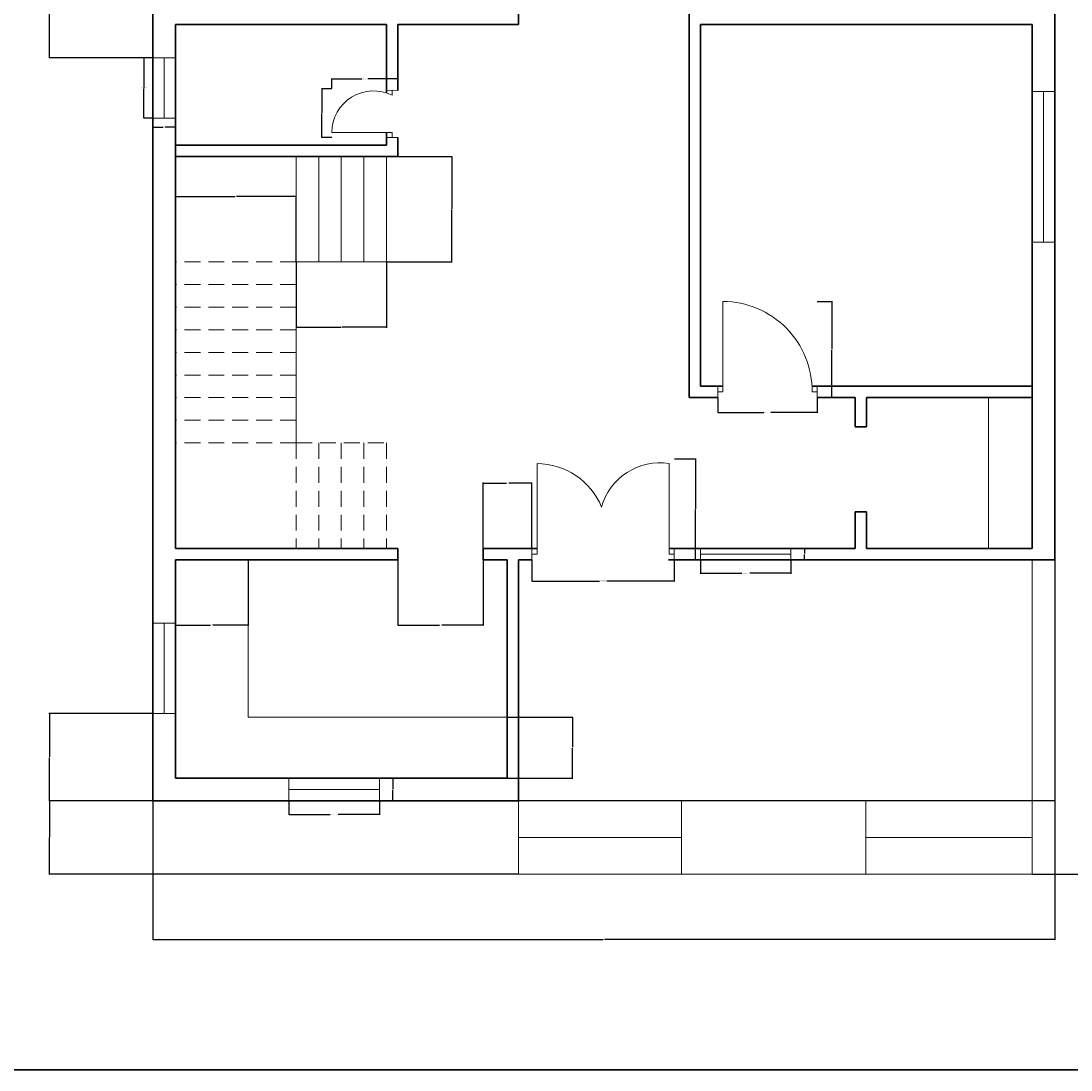
# Model space of a CAD drawing. Units: inches. Extents: x 1832 to 2989, y 1644 to 2902.
# Tile 4 of 8: x 2343 to 2760, y 1644 to 2061. Entities that reach past the tile are written whole.
import ezdxf

# ---------------------------------------------------------------- set-up
doc = ezdxf.new("R2010")
doc.units = ezdxf.units.IN
doc.linetypes.add('DASHED2', pattern=[9.525, 6.35, -3.175])
for name, color, linetype, lineweight in [('A-ANNO-DIMS', 2, 'Continuous', 18), ('A-ANNO-TTLB', 7, 'Continuous', 35), ('A-DOOR', 3, 'Continuous', 18), ('A-FLOR', 7, 'Continuous', 25), ('A-FLOR-CASE', 8, 'Continuous', 18), ('A-FLOR-STRS', 7, 'Continuous', 18), ('A-FLOR-STRS-OVHD', 254, 'DASHED2', 13), ('A-GLAZ', 4, 'Continuous', 18), ('A-WALL', 7, 'Continuous', 35)]:
    doc.layers.add(name, color=color, linetype=linetype, lineweight=lineweight)
doc.styles.get("Standard").update_dxf_attribs({"font": 'arial.ttf'})
doc.dimstyles.get("Standard").update_dxf_attribs({"dimtxt": 0.18, "dimasz": 0.18, "dimexe": 0.18, "dimexo": 0.0625, "dimgap": 0.09, "dimtad": 0, "dimtih": 1, "dimtoh": 1, "dimdec": 4, "dimzin": 0, "dimdsep": 46, "dimtxsty": 'Standard', "dimcen": 0.09, "dimadec": 0, "dimazin": 0, "dimtfac": 1, "dimtdec": 4, "dimtofl": 0, "dimtmove": 0, "dimatfit": 3, "dimfxl": 1, "dimtolj": 1, "dimtzin": 0, "dimarcsym": 0})

# ---------------------------------------------------------------- blocks, each defined once
blk = doc.blocks.new('WIN-PLAN-60IN')
for p, q in [((0, 9), (0, 0)), ((60, 4.5), (60, 9)), ((60, 9), (60, 0)), ((0, 0), (0, 4.5)), ((0, 4.5), (60, 4.5))]:
    blk.add_line(p, q)
blk = doc.blocks.new('WIN-PLAN-24IN')
for p, q in [((0, 9), (0, 0)), ((24, 4.5), (24, 9)), ((24, 9), (24, 0)), ((0, 0), (0, 4.5)), ((0, 4.5), (24, 4.5))]:
    blk.add_line(p, q)
blk = doc.blocks.new('WIN-PLAN-36IN')
for p, q in [((0, 9), (0, 0)), ((36, 4.5), (36, 9)), ((36, 9), (36, 0)), ((0, 0), (0, 4.5)), ((0, 4.5), (36, 4.5))]:
    blk.add_line(p, q)
blk = doc.blocks.new('WIN-PLAN-36IN-2')
for p, q in [((0, 36), (9, 36)), ((9, 36), (4.5, 36)), ((4.5, 36), (4.5, 0)), ((9, 0), (0, 0)), ((4.5, 0), (9, 0))]:
    blk.add_line(p, q)
blk = doc.blocks.new('DOOR-PLAN-WC')
for p, q in [((21.75, 18.87), (26.25, 18.72)), ((26.25, 18.72), (24, 18.8)), ((24, 18.8), (24, 16.8)), ((24, 2), (0, 2)), ((21.75, 0), (26.25, 0)), ((24, 0), (24, 2)), ((26.25, 0), (24, 0))]:
    blk.add_line(p, q)
blk.add_arc((16.56, 2), 16.56, 63.308, 180)
blk = doc.blocks.new('DOOR-PLAN-ENTRY-PAIR')
for p, q in [((2, 2.25), (2, 38.25)), ((54.64, 2.25), (54.64, 38.25)), ((0, 4.5), (0, 0)), ((56.64, 4.5), (56.64, 0)), ((56.64, 4.5), (56.64, 2.25)), ((0, 2.25), (2, 2.25)), ((56.64, 2.25), (54.64, 2.25)), ((56.64, 0), (56.64, 2.25))]:
    blk.add_line(p, q)
for centre, radius, start, end in [((2, 10.56), 27.69, 21.9895, 90), ((50.82, 14.55), 24, 80.8436, 164.5954)]:
    blk.add_arc(centre, radius, start, end)
blk = doc.blocks.new('DOOR-PLAN-LIVING')
for p, q in [((2, 26.25), (2, 38.25)), ((2, 2.25), (2, 26.25)), ((0, 4.5), (0, 0)), ((39.53, 4.5), (39.53, 0)), ((0, 0), (0, 2.25)), ((0, 2.25), (2, 2.25)), ((39.53, 2.25), (37.53, 2.25)), ((39.53, 0), (39.53, 2.25))]:
    blk.add_line(p, q)
blk.add_arc((2, 2.72), 35.53, 359.2416, 90)
blk = doc.blocks.new('WIN-PLAN-PARTITION-36IN')
for p, q in [((0, 4.5), (0, 0)), ((36, 2.25), (36, 4.5)), ((36, 4.5), (36, 0)), ((0, 2.25), (36, 2.25))]:
    blk.add_line(p, q)
blk = doc.blocks.new('*D43')
at = {"layer": 'A-ANNO-DIMS', "color": 0, "lineweight": -2, "transparency": 16777216}
for p, q in [((2466.29, 2034.14), (2466.29, 2038.19)), ((2466.47, 2038.01), (2478.22, 2038.01)), ((2492.36, 2038.01), (2480.6, 2038.01)), ((2492.54, 2034.14), (2492.54, 2038.19))]:
    blk.add_line(p, q, dxfattribs=at)
at = {"layer": 'A-ANNO-DIMS', "color": 0, "transparency": 16777216}
for points in [[(2466.47, 2038.04), (2466.47, 2037.98), (2466.29, 2038.01)], [(2492.36, 2038.04), (2492.36, 2037.98), (2492.54, 2038.01)]]:
    blk.add_solid(points, dxfattribs=at)
at = {"layer": 'Defpoints', "color": 0, "transparency": 16777216}
for p in [(2492.54, 2038.01), (2466.29, 2034.08), (2492.54, 2034.08)]:
    blk.add_point(p, dxfattribs=at)
at = {"layer": 'A-ANNO-DIMS', "color": 0, "transparency": 16777216, "insert": (2479.41, 2038.01), "char_height": 0.18, "attachment_point": 5}
blk.add_mtext('\\A1;WC DOOR 26 TYP.', dxfattribs=at)
blk = doc.blocks.new('*D44')
at = {"layer": 'A-ANNO-DIMS', "color": 0, "lineweight": -2, "transparency": 16777216}
for p, q in [((2466.22, 2034.08), (2462.17, 2034.08)), ((2462.35, 2033.9), (2462.35, 2024.57)), ((2462.35, 2014.88), (2462.35, 2024.21)), ((2466.22, 2014.7), (2462.17, 2014.7))]:
    blk.add_line(p, q, dxfattribs=at)
at = {"layer": 'A-ANNO-DIMS', "color": 0, "transparency": 16777216}
for points in [[(2462.32, 2033.9), (2462.38, 2033.9), (2462.35, 2034.08)], [(2462.32, 2014.88), (2462.38, 2014.88), (2462.35, 2014.7)]]:
    blk.add_solid(points, dxfattribs=at)
at = {"layer": 'Defpoints', "color": 0, "transparency": 16777216}
for p in [(2462.35, 2034.08), (2466.29, 2034.08), (2466.29, 2014.7)]:
    blk.add_point(p, dxfattribs=at)
at = {"layer": 'A-ANNO-DIMS', "color": 0, "transparency": 16777216, "insert": (2462.35, 2024.39), "char_height": 0.18, "attachment_point": 5}
blk.add_mtext('\\A1;19 TYP.', dxfattribs=at)
blk = doc.blocks.new('*D45')
at = {"layer": 'A-ANNO-DIMS', "color": 0, "lineweight": -2, "transparency": 16777216}
for p, q in [((2619.9, 1911.11), (2619.9, 1905.06)), ((2659.42, 1911.11), (2659.42, 1905.06)), ((2620.08, 1905.24), (2638.28, 1905.24)), ((2659.24, 1905.24), (2641.04, 1905.24))]:
    blk.add_line(p, q, dxfattribs=at)
at = {"layer": 'A-ANNO-DIMS', "color": 0, "transparency": 16777216}
for points in [[(2620.08, 1905.27), (2620.08, 1905.21), (2619.9, 1905.24)], [(2659.24, 1905.27), (2659.24, 1905.21), (2659.42, 1905.24)]]:
    blk.add_solid(points, dxfattribs=at)
at = {"layer": 'Defpoints', "color": 0, "transparency": 16777216}
for p in [(2619.9, 1911.17), (2659.42, 1911.17), (2659.42, 1905.24)]:
    blk.add_point(p, dxfattribs=at)
at = {"layer": 'A-ANNO-DIMS', "color": 0, "transparency": 16777216, "insert": (2639.66, 1905.24), "char_height": 0.18, "attachment_point": 5}
blk.add_mtext('\\A1;LIVING DOOR 40 TYP.', dxfattribs=at)
blk = doc.blocks.new('*D46')
at = {"layer": 'A-ANNO-DIMS', "color": 0, "lineweight": -2, "transparency": 16777216}
for p, q in [((2659.49, 1949.42), (2665.53, 1949.42)), ((2665.35, 1949.24), (2665.35, 1930.48)), ((2665.35, 1911.35), (2665.35, 1930.12)), ((2659.49, 1911.17), (2665.53, 1911.17))]:
    blk.add_line(p, q, dxfattribs=at)
at = {"layer": 'A-ANNO-DIMS', "color": 0, "transparency": 16777216}
for points in [[(2665.32, 1949.24), (2665.38, 1949.24), (2665.35, 1949.42)], [(2665.32, 1911.35), (2665.38, 1911.35), (2665.35, 1911.17)]]:
    blk.add_solid(points, dxfattribs=at)
at = {"layer": 'Defpoints', "color": 0, "transparency": 16777216}
for p in [(2659.42, 1949.42), (2665.35, 1949.42), (2659.42, 1911.17)]:
    blk.add_point(p, dxfattribs=at)
at = {"layer": 'A-ANNO-DIMS', "color": 0, "transparency": 16777216, "insert": (2665.35, 1930.3), "char_height": 0.18, "attachment_point": 5}
blk.add_mtext('\\A1;38 TYP.', dxfattribs=at)
blk = doc.blocks.new('*D47')
at = {"layer": 'A-ANNO-DIMS', "color": 0, "lineweight": -2, "transparency": 16777216}
for p, q in [((2545.94, 1846.61), (2545.94, 1838)), ((2602.58, 1846.61), (2602.58, 1838)), ((2546.12, 1838.18), (2572.77, 1838.18)), ((2602.4, 1838.18), (2575.75, 1838.18))]:
    blk.add_line(p, q, dxfattribs=at)
at = {"layer": 'A-ANNO-DIMS', "color": 0, "transparency": 16777216}
for points in [[(2546.12, 1838.21), (2546.12, 1838.15), (2545.94, 1838.18)], [(2602.4, 1838.21), (2602.4, 1838.15), (2602.58, 1838.18)]]:
    blk.add_solid(points, dxfattribs=at)
at = {"layer": 'Defpoints', "color": 0, "transparency": 16777216}
for p in [(2545.94, 1846.67), (2602.58, 1846.67), (2602.58, 1838.18)]:
    blk.add_point(p, dxfattribs=at)
at = {"layer": 'A-ANNO-DIMS', "color": 0, "transparency": 16777216, "insert": (2574.26, 1838.18), "char_height": 0.18, "attachment_point": 5}
blk.add_mtext('\\A1;PAIRED ENTRY 57 TYP.', dxfattribs=at)
blk = doc.blocks.new('*D48')
at = {"layer": 'A-ANNO-DIMS', "color": 0, "lineweight": -2, "transparency": 16777216}
for p, q in [((2602.64, 1886.87), (2611.26, 1886.87)), ((2611.08, 1886.69), (2611.08, 1866.95)), ((2611.08, 1846.85), (2611.08, 1866.59)), ((2602.64, 1846.67), (2611.26, 1846.67))]:
    blk.add_line(p, q, dxfattribs=at)
at = {"layer": 'A-ANNO-DIMS', "color": 0, "transparency": 16777216}
for points in [[(2611.05, 1886.69), (2611.11, 1886.69), (2611.08, 1886.87)], [(2611.05, 1846.85), (2611.11, 1846.85), (2611.08, 1846.67)]]:
    blk.add_solid(points, dxfattribs=at)
at = {"layer": 'Defpoints', "color": 0, "transparency": 16777216}
for p in [(2602.58, 1886.87), (2611.08, 1886.87), (2602.58, 1846.67)]:
    blk.add_point(p, dxfattribs=at)
at = {"layer": 'A-ANNO-DIMS', "color": 0, "transparency": 16777216, "insert": (2611.08, 1866.77), "char_height": 0.18, "attachment_point": 5}
blk.add_mtext('\\A1;40 TYP.', dxfattribs=at)
blk = doc.blocks.new('*D53')
at = {"layer": 'A-ANNO-DIMS', "color": 0, "lineweight": -2, "transparency": 16777216}
for p, q in [((2394.97, 2046.39), (2391.26, 2046.39)), ((2391.44, 2046.21), (2391.44, 2034.57)), ((2391.44, 2022.57), (2391.44, 2034.2)), ((2394.97, 2022.39), (2391.26, 2022.39))]:
    blk.add_line(p, q, dxfattribs=at)
at = {"layer": 'A-ANNO-DIMS', "color": 0, "transparency": 16777216}
for points in [[(2391.41, 2046.21), (2391.47, 2046.21), (2391.44, 2046.39)], [(2391.41, 2022.57), (2391.47, 2022.57), (2391.44, 2022.39)]]:
    blk.add_solid(points, dxfattribs=at)
at = {"layer": 'Defpoints', "color": 0, "transparency": 16777216}
for p in [(2395.04, 2046.39), (2391.44, 2022.39), (2395.04, 2022.39)]:
    blk.add_point(p, dxfattribs=at)
at = {"layer": 'A-ANNO-DIMS', "color": 0, "transparency": 16777216, "insert": (2391.44, 2034.39), "char_height": 0.18, "attachment_point": 5}
blk.add_mtext('\\A1;WC WINDOW 24 TYP.', dxfattribs=at)
blk = doc.blocks.new('*D54')
at = {"layer": 'A-ANNO-DIMS', "color": 0, "lineweight": -2, "transparency": 16777216}
for p, q in [((2395.04, 2022.32), (2395.04, 2018.61)), ((2395.22, 2018.79), (2399.08, 2018.79)), ((2403.86, 2018.79), (2399.99, 2018.79)), ((2404.04, 2022.32), (2404.04, 2018.61))]:
    blk.add_line(p, q, dxfattribs=at)
at = {"layer": 'A-ANNO-DIMS', "color": 0, "transparency": 16777216}
for points in [[(2395.22, 2018.82), (2395.22, 2018.76), (2395.04, 2018.79)], [(2403.86, 2018.82), (2403.86, 2018.76), (2404.04, 2018.79)]]:
    blk.add_solid(points, dxfattribs=at)
at = {"layer": 'Defpoints', "color": 0, "transparency": 16777216}
for p in [(2395.04, 2022.39), (2404.04, 2022.39), (2404.04, 2018.79)]:
    blk.add_point(p, dxfattribs=at)
at = {"layer": 'A-ANNO-DIMS', "color": 0, "transparency": 16777216, "insert": (2399.54, 2018.79), "char_height": 0.18, "attachment_point": 5}
blk.add_mtext('\\A1;9 TYP.', dxfattribs=at)
blk = doc.blocks.new('*D55')
at = {"layer": 'A-ANNO-DIMS', "color": 0, "lineweight": -2, "transparency": 16777216}
for p, q in [((2449.19, 1750.61), (2449.19, 1745.09)), ((2485.19, 1750.61), (2485.19, 1745.09)), ((2449.37, 1745.27), (2465.61, 1745.27)), ((2485.01, 1745.27), (2468.76, 1745.27))]:
    blk.add_line(p, q, dxfattribs=at)
at = {"layer": 'A-ANNO-DIMS', "color": 0, "transparency": 16777216}
for points in [[(2449.37, 1745.3), (2449.37, 1745.24), (2449.19, 1745.27)], [(2485.01, 1745.3), (2485.01, 1745.24), (2485.19, 1745.27)]]:
    blk.add_solid(points, dxfattribs=at)
at = {"layer": 'Defpoints', "color": 0, "transparency": 16777216}
for p in [(2449.19, 1750.67), (2485.19, 1750.67), (2449.19, 1745.27)]:
    blk.add_point(p, dxfattribs=at)
at = {"layer": 'A-ANNO-DIMS', "color": 0, "transparency": 16777216, "insert": (2467.19, 1745.27), "char_height": 0.18, "attachment_point": 5}
blk.add_mtext('\\A1;FRONT WINDOW 36 TYP.', dxfattribs=at)
blk = doc.blocks.new('*D56')
at = {"layer": 'A-ANNO-DIMS', "color": 0, "lineweight": -2, "transparency": 16777216}
for p, q in [((2485.25, 1759.67), (2490.77, 1759.67)), ((2490.59, 1759.49), (2490.59, 1755.35)), ((2490.59, 1750.85), (2490.59, 1754.99)), ((2485.25, 1750.67), (2490.77, 1750.67))]:
    blk.add_line(p, q, dxfattribs=at)
at = {"layer": 'A-ANNO-DIMS', "color": 0, "transparency": 16777216}
for points in [[(2490.56, 1759.49), (2490.62, 1759.49), (2490.59, 1759.67)], [(2490.56, 1750.85), (2490.62, 1750.85), (2490.59, 1750.67)]]:
    blk.add_solid(points, dxfattribs=at)
at = {"layer": 'Defpoints', "color": 0, "transparency": 16777216}
for p in [(2485.19, 1759.67), (2485.19, 1750.67), (2490.59, 1750.67)]:
    blk.add_point(p, dxfattribs=at)
at = {"layer": 'A-ANNO-DIMS', "color": 0, "transparency": 16777216, "insert": (2490.59, 1755.17), "char_height": 0.18, "attachment_point": 5}
blk.add_mtext('\\A1;9 TYP.', dxfattribs=at)
blk = doc.blocks.new('*D59')
at = {"layer": 'A-ANNO-DIMS', "color": 0, "lineweight": -2, "transparency": 16777216}
for p, q in [((2613.04, 1846.61), (2613.04, 1841.09)), ((2649.04, 1846.61), (2649.04, 1841.09)), ((2613.22, 1841.27), (2629.43, 1841.27)), ((2648.86, 1841.27), (2632.65, 1841.27))]:
    blk.add_line(p, q, dxfattribs=at)
at = {"layer": 'A-ANNO-DIMS', "color": 0, "transparency": 16777216}
for points in [[(2613.22, 1841.3), (2613.22, 1841.24), (2613.04, 1841.27)], [(2648.86, 1841.3), (2648.86, 1841.24), (2649.04, 1841.27)]]:
    blk.add_solid(points, dxfattribs=at)
at = {"layer": 'Defpoints', "color": 0, "transparency": 16777216}
for p in [(2613.04, 1846.67), (2649.04, 1846.67), (2649.04, 1841.27)]:
    blk.add_point(p, dxfattribs=at)
at = {"layer": 'A-ANNO-DIMS', "color": 0, "transparency": 16777216, "insert": (2631.04, 1841.27), "char_height": 0.18, "attachment_point": 5}
blk.add_mtext('\\A1;SITOUT WINDOW 36 TYP.', dxfattribs=at)
blk = doc.blocks.new('*D60')
at = {"layer": 'A-ANNO-DIMS', "color": 0, "lineweight": -2, "transparency": 16777216}
for p, q in [((2649.1, 1851.17), (2654.62, 1851.17)), ((2654.44, 1850.99), (2654.44, 1849.1)), ((2654.44, 1846.85), (2654.44, 1848.74)), ((2649.1, 1846.67), (2654.62, 1846.67))]:
    blk.add_line(p, q, dxfattribs=at)
at = {"layer": 'A-ANNO-DIMS', "color": 0, "transparency": 16777216}
for points in [[(2654.41, 1850.99), (2654.47, 1850.99), (2654.44, 1851.17)], [(2654.41, 1846.85), (2654.47, 1846.85), (2654.44, 1846.67)]]:
    blk.add_solid(points, dxfattribs=at)
at = {"layer": 'Defpoints', "color": 0, "transparency": 16777216}
for p in [(2649.04, 1851.17), (2654.44, 1851.17), (2649.04, 1846.67)]:
    blk.add_point(p, dxfattribs=at)
at = {"layer": 'A-ANNO-DIMS', "color": 0, "transparency": 16777216, "insert": (2654.44, 1848.92), "char_height": 0.18, "attachment_point": 5}
blk.add_mtext('\\A1;5 TYP.', dxfattribs=at)
blk = doc.blocks.new('*D81')
at = {"layer": 'A-ANNO-DIMS', "color": 0, "lineweight": -2, "transparency": 16777216}
for p, q in [((2395.04, 1750.61), (2395.04, 1695.34)), ((2754.04, 1750.61), (2754.04, 1695.34)), ((2395.22, 1695.52), (2574.25, 1695.52)), ((2753.86, 1695.52), (2574.82, 1695.52))]:
    blk.add_line(p, q, dxfattribs=at)
at = {"layer": 'A-ANNO-DIMS', "color": 0, "transparency": 16777216}
for points in [[(2395.22, 1695.55), (2395.22, 1695.49), (2395.04, 1695.52)], [(2753.86, 1695.55), (2753.86, 1695.49), (2754.04, 1695.52)]]:
    blk.add_solid(points, dxfattribs=at)
at = {"layer": 'Defpoints', "color": 0, "transparency": 16777216}
for p in [(2395.04, 1750.67), (2754.04, 1750.67), (2754.04, 1695.52)]:
    blk.add_point(p, dxfattribs=at)
at = {"layer": 'A-ANNO-DIMS', "color": 0, "transparency": 16777216, "insert": (2574.54, 1695.52), "char_height": 0.18, "attachment_point": 5}
blk.add_mtext('\\A1;359', dxfattribs=at)
blk = doc.blocks.new('*D82')
at = {"layer": 'A-ANNO-DIMS', "color": 0, "lineweight": -2, "transparency": 16777216}
for p, q in [((2754.1, 2229.17), (2811, 2229.17)), ((2810.82, 2228.99), (2810.82, 1975.53)), ((2810.82, 1721.7), (2810.82, 1975.17)), ((2745.1, 1721.52), (2811, 1721.52))]:
    blk.add_line(p, q, dxfattribs=at)
at = {"layer": 'A-ANNO-DIMS', "color": 0, "transparency": 16777216}
for points in [[(2810.79, 2228.99), (2810.85, 2228.99), (2810.82, 2229.17)], [(2810.79, 1721.7), (2810.85, 1721.7), (2810.82, 1721.52)]]:
    blk.add_solid(points, dxfattribs=at)
at = {"layer": 'Defpoints', "color": 0, "transparency": 16777216}
for p in [(2754.04, 2229.17), (2810.82, 2229.17), (2745.04, 1721.52)]:
    blk.add_point(p, dxfattribs=at)
at = {"layer": 'A-ANNO-DIMS', "color": 0, "transparency": 16777216, "insert": (2810.82, 1975.35), "char_height": 0.18, "attachment_point": 5}
blk.add_mtext('\\A1;507.6', dxfattribs=at)
blk = doc.blocks.new('*D83')
at = {"layer": 'A-ANNO-DIMS', "color": 0, "lineweight": -2, "transparency": 16777216}
for p, q in [((2540.47, 1750.67), (2353.64, 1750.67)), ((2353.82, 1750.49), (2353.82, 1736.28)), ((2353.82, 1721.7), (2353.82, 1735.92)), ((2540.47, 1721.52), (2353.64, 1721.52))]:
    blk.add_line(p, q, dxfattribs=at)
at = {"layer": 'A-ANNO-DIMS', "color": 0, "transparency": 16777216}
for points in [[(2353.79, 1750.49), (2353.85, 1750.49), (2353.82, 1750.67)], [(2353.79, 1721.7), (2353.85, 1721.7), (2353.82, 1721.52)]]:
    blk.add_solid(points, dxfattribs=at)
at = {"layer": 'Defpoints', "color": 0, "transparency": 16777216}
for p in [(2540.54, 1750.67), (2353.82, 1721.52), (2540.54, 1721.52)]:
    blk.add_point(p, dxfattribs=at)
at = {"layer": 'A-ANNO-DIMS', "color": 0, "transparency": 16777216, "insert": (2353.82, 1736.1), "char_height": 0.18, "attachment_point": 5}
blk.add_mtext('\\A1;29.15', dxfattribs=at)
blk = doc.blocks.new('*D84')
at = {"layer": 'A-ANNO-DIMS', "color": 0, "lineweight": -2, "transparency": 16777216}
for p, q in [((2394.97, 1785.42), (2353.64, 1785.42)), ((2353.82, 1785.24), (2353.82, 1768.23)), ((2353.82, 1750.85), (2353.82, 1767.86)), ((2394.97, 1750.67), (2353.64, 1750.67))]:
    blk.add_line(p, q, dxfattribs=at)
at = {"layer": 'A-ANNO-DIMS', "color": 0, "transparency": 16777216}
for points in [[(2353.79, 1785.24), (2353.85, 1785.24), (2353.82, 1785.42)], [(2353.79, 1750.85), (2353.85, 1750.85), (2353.82, 1750.67)]]:
    blk.add_solid(points, dxfattribs=at)
at = {"layer": 'Defpoints', "color": 0, "transparency": 16777216}
for p in [(2353.82, 1785.42), (2395.04, 1785.42), (2395.04, 1750.67)]:
    blk.add_point(p, dxfattribs=at)
at = {"layer": 'A-ANNO-DIMS', "color": 0, "transparency": 16777216, "insert": (2353.82, 1768.04), "char_height": 0.18, "attachment_point": 5}
blk.add_mtext('\\A1;34.74', dxfattribs=at)
blk = doc.blocks.new('*D85')
at = {"layer": 'A-ANNO-DIMS', "color": 0, "lineweight": -2, "transparency": 16777216}
for p, q in [((2379.76, 2112.91), (2353.64, 2112.91)), ((2353.82, 2112.73), (2353.82, 2079.83)), ((2353.82, 2046.57), (2353.82, 2079.47)), ((2394.97, 2046.39), (2353.64, 2046.39))]:
    blk.add_line(p, q, dxfattribs=at)
at = {"layer": 'A-ANNO-DIMS', "color": 0, "transparency": 16777216}
for points in [[(2353.79, 2112.73), (2353.85, 2112.73), (2353.82, 2112.91)], [(2353.79, 2046.57), (2353.85, 2046.57), (2353.82, 2046.39)]]:
    blk.add_solid(points, dxfattribs=at)
at = {"layer": 'Defpoints', "color": 0, "transparency": 16777216}
for p in [(2353.82, 2112.91), (2379.82, 2112.91), (2395.04, 2046.39)]:
    blk.add_point(p, dxfattribs=at)
at = {"layer": 'A-ANNO-DIMS', "color": 0, "transparency": 16777216, "insert": (2353.82, 2079.65), "char_height": 0.18, "attachment_point": 5}
blk.add_mtext('\\A1;66.53', dxfattribs=at)
blk = doc.blocks.new('*D91')
at = {"layer": 'A-ANNO-DIMS', "color": 0, "lineweight": -2, "transparency": 16777216}
for p, q in [((2452.04, 1965.11), (2452.04, 1938.99)), ((2488.04, 1965.11), (2488.04, 1938.99)), ((2452.22, 1939.17), (2469.82, 1939.17)), ((2487.86, 1939.17), (2470.25, 1939.17))]:
    blk.add_line(p, q, dxfattribs=at)
at = {"layer": 'A-ANNO-DIMS', "color": 0, "transparency": 16777216}
for points in [[(2452.22, 1939.2), (2452.22, 1939.14), (2452.04, 1939.17)], [(2487.86, 1939.2), (2487.86, 1939.14), (2488.04, 1939.17)]]:
    blk.add_solid(points, dxfattribs=at)
at = {"layer": 'Defpoints', "color": 0, "transparency": 16777216}
for p in [(2452.04, 1965.17), (2488.04, 1965.17), (2452.04, 1939.17)]:
    blk.add_point(p, dxfattribs=at)
at = {"layer": 'A-ANNO-DIMS', "color": 0, "transparency": 16777216, "insert": (2470.04, 1939.17), "char_height": 0.18, "attachment_point": 5}
blk.add_mtext('\\A1;36', dxfattribs=at)
blk = doc.blocks.new('*D92')
at = {"layer": 'A-ANNO-DIMS', "color": 0, "lineweight": -2, "transparency": 16777216}
for p, q in [((2488.1, 2007.17), (2514.22, 2007.17)), ((2514.04, 2006.99), (2514.04, 1986.35)), ((2514.04, 1965.35), (2514.04, 1985.99)), ((2488.1, 1965.17), (2514.22, 1965.17))]:
    blk.add_line(p, q, dxfattribs=at)
at = {"layer": 'A-ANNO-DIMS', "color": 0, "transparency": 16777216}
for points in [[(2514.01, 2006.99), (2514.07, 2006.99), (2514.04, 2007.17)], [(2514.01, 1965.35), (2514.07, 1965.35), (2514.04, 1965.17)]]:
    blk.add_solid(points, dxfattribs=at)
at = {"layer": 'Defpoints', "color": 0, "transparency": 16777216}
for p in [(2488.04, 2007.17), (2488.04, 1965.17), (2514.04, 1965.17)]:
    blk.add_point(p, dxfattribs=at)
at = {"layer": 'A-ANNO-DIMS', "color": 0, "transparency": 16777216, "insert": (2514.04, 1986.17), "char_height": 0.18, "attachment_point": 5}
blk.add_mtext('\\A1;42', dxfattribs=at)
blk = doc.blocks.new('*D93')
at = {"layer": 'A-ANNO-DIMS', "color": 0, "lineweight": -2, "transparency": 16777216}
for p, q in [((2404.04, 1965.24), (2404.04, 1991.35)), ((2404.22, 1991.17), (2427.81, 1991.17)), ((2451.86, 1991.17), (2428.26, 1991.17)), ((2452.04, 1965.24), (2452.04, 1991.35))]:
    blk.add_line(p, q, dxfattribs=at)
at = {"layer": 'A-ANNO-DIMS', "color": 0, "transparency": 16777216}
for points in [[(2404.22, 1991.2), (2404.22, 1991.14), (2404.04, 1991.17)], [(2451.86, 1991.2), (2451.86, 1991.14), (2452.04, 1991.17)]]:
    blk.add_solid(points, dxfattribs=at)
at = {"layer": 'Defpoints', "color": 0, "transparency": 16777216}
for p in [(2452.04, 1991.17), (2404.04, 1965.17), (2452.04, 1965.17)]:
    blk.add_point(p, dxfattribs=at)
at = {"layer": 'A-ANNO-DIMS', "color": 0, "transparency": 16777216, "insert": (2428.04, 1991.17), "char_height": 0.18, "attachment_point": 5}
blk.add_mtext('\\A1;48', dxfattribs=at)
blk = doc.blocks.new('*D94')
at = {"layer": 'A-ANNO-DIMS', "color": 0, "lineweight": -2, "transparency": 16777216}
for p, q in [((2404.04, 1846.61), (2404.04, 1820.49)), ((2432.9, 1846.61), (2432.9, 1820.49)), ((2404.22, 1820.67), (2418, 1820.67)), ((2432.72, 1820.67), (2418.93, 1820.67))]:
    blk.add_line(p, q, dxfattribs=at)
at = {"layer": 'A-ANNO-DIMS', "color": 0, "transparency": 16777216}
for points in [[(2404.22, 1820.7), (2404.22, 1820.64), (2404.04, 1820.67)], [(2432.72, 1820.7), (2432.72, 1820.64), (2432.9, 1820.67)]]:
    blk.add_solid(points, dxfattribs=at)
at = {"layer": 'Defpoints', "color": 0, "transparency": 16777216}
for p in [(2404.04, 1846.67), (2432.9, 1846.67), (2404.04, 1820.67)]:
    blk.add_point(p, dxfattribs=at)
at = {"layer": 'A-ANNO-DIMS', "color": 0, "transparency": 16777216, "insert": (2418.47, 1820.67), "char_height": 0.18, "attachment_point": 5}
blk.add_mtext('\\A1;28.864', dxfattribs=at)
blk = doc.blocks.new('*D95')
at = {"layer": 'A-ANNO-DIMS', "color": 0, "lineweight": -2, "transparency": 16777216}
for p, q in [((2536.1, 1784.05), (2562.22, 1784.05)), ((2562.04, 1783.87), (2562.04, 1772.05)), ((2562.04, 1759.85), (2562.04, 1771.68)), ((2536.1, 1759.67), (2562.22, 1759.67))]:
    blk.add_line(p, q, dxfattribs=at)
at = {"layer": 'A-ANNO-DIMS', "color": 0, "transparency": 16777216}
for points in [[(2562.01, 1783.87), (2562.07, 1783.87), (2562.04, 1784.05)], [(2562.01, 1759.85), (2562.07, 1759.85), (2562.04, 1759.67)]]:
    blk.add_solid(points, dxfattribs=at)
at = {"layer": 'Defpoints', "color": 0, "transparency": 16777216}
for p in [(2536.04, 1784.05), (2536.04, 1759.67), (2562.04, 1759.67)]:
    blk.add_point(p, dxfattribs=at)
at = {"layer": 'A-ANNO-DIMS', "color": 0, "transparency": 16777216, "insert": (2562.04, 1771.86), "char_height": 0.18, "attachment_point": 5}
blk.add_mtext('\\A1;24.38', dxfattribs=at)
blk = doc.blocks.new('*D96')
at = {"layer": 'A-ANNO-DIMS', "color": 0, "lineweight": -2, "transparency": 16777216}
for p, q in [((2492.54, 1846.61), (2492.54, 1820.49)), ((2526.57, 1846.61), (2526.57, 1820.49)), ((2492.72, 1820.67), (2509.09, 1820.67)), ((2526.39, 1820.67), (2510.02, 1820.67))]:
    blk.add_line(p, q, dxfattribs=at)
at = {"layer": 'A-ANNO-DIMS', "color": 0, "transparency": 16777216}
for points in [[(2492.72, 1820.7), (2492.72, 1820.64), (2492.54, 1820.67)], [(2526.39, 1820.7), (2526.39, 1820.64), (2526.57, 1820.67)]]:
    blk.add_solid(points, dxfattribs=at)
at = {"layer": 'Defpoints', "color": 0, "transparency": 16777216}
for p in [(2492.54, 1846.67), (2526.57, 1846.67), (2492.54, 1820.67)]:
    blk.add_point(p, dxfattribs=at)
at = {"layer": 'A-ANNO-DIMS', "color": 0, "transparency": 16777216, "insert": (2509.55, 1820.67), "char_height": 0.18, "attachment_point": 5}
blk.add_mtext('\\A1;34.034', dxfattribs=at)
blk = doc.blocks.new('*D97')
at = {"layer": 'A-ANNO-DIMS', "color": 0, "lineweight": -2, "transparency": 16777216}
for p, q in [((2526.57, 1851.24), (2526.57, 1877.35)), ((2526.75, 1877.17), (2535.8, 1877.17)), ((2545.76, 1877.17), (2536.71, 1877.17)), ((2545.94, 1851.24), (2545.94, 1877.35))]:
    blk.add_line(p, q, dxfattribs=at)
at = {"layer": 'A-ANNO-DIMS', "color": 0, "transparency": 16777216}
for points in [[(2526.75, 1877.2), (2526.75, 1877.14), (2526.57, 1877.17)], [(2545.76, 1877.2), (2545.76, 1877.14), (2545.94, 1877.17)]]:
    blk.add_solid(points, dxfattribs=at)
at = {"layer": 'Defpoints', "color": 0, "transparency": 16777216}
for p in [(2545.94, 1877.17), (2526.57, 1851.17), (2545.94, 1851.17)]:
    blk.add_point(p, dxfattribs=at)
at = {"layer": 'A-ANNO-DIMS', "color": 0, "transparency": 16777216, "insert": (2536.26, 1877.17), "char_height": 0.18, "attachment_point": 5}
blk.add_mtext('\\A1;19.372', dxfattribs=at)

msp = doc.modelspace()

# ---------------------------------------------------------------- linework, layer by layer
at = {"layer": 'A-ANNO-TTLB'}
msp.add_lwpolyline([(1831.6677, 2901.9044), (2988.9144, 2901.9044), (2988.9144, 1643.5851), (1831.6677, 1643.5851)], close=True, dxfattribs=at)
at = {"layer": 'A-FLOR'}
for p, q in [((2754.0354, 1846.6726), (2754.0354, 1750.6726)), ((2754.0354, 1750.6726), (2540.5354, 1750.6726))]:
    msp.add_line(p, q, dxfattribs=at)
at = {"layer": 'A-FLOR-CASE'}
for p, q in [((2727.6602, 1911.1726), (2727.6602, 1851.1726)), ((2432.899, 1846.6726), (2432.899, 1784.0547)), ((2432.899, 1784.0547), (2536.0354, 1784.0547))]:
    msp.add_line(p, q, dxfattribs=at)
at = {"layer": 'A-FLOR-STRS'}
for p, q in [((2404.0354, 2007.1726), (2452.0354, 2007.1726)), ((2452.0354, 2007.1726), (2452.0354, 1959.1726)), ((2452.0354, 2007.1726), (2452.0354, 1965.1726)), ((2461.0354, 2007.1726), (2461.0354, 1965.1726)), ((2470.0354, 2007.1726), (2470.0354, 1965.1726)), ((2479.0354, 2007.1726), (2479.0354, 1965.1726)), ((2488.0354, 2007.1726), (2488.0354, 1965.1726)), ((2452.0354, 1965.1726), (2488.0354, 1965.1726)), ((2452.0354, 1959.1726), (2452.0354, 1893.1726)), ((2745.0354, 1846.6726), (2745.0354, 1721.5243)), ((2540.5354, 1750.6726), (2540.5354, 1721.5243)), ((2605.5218, 1750.6726), (2605.5218, 1721.5243)), ((2678.784, 1721.5243), (2678.784, 1750.6726)), ((2540.5354, 1736.0984), (2605.5218, 1736.0984)), ((2678.784, 1736.0984), (2745.0354, 1736.0984)), ((2540.5354, 1721.5243), (2745.0354, 1721.5243)), ((2605.5218, 1721.5243), (2678.784, 1721.5243))]:
    msp.add_line(p, q, dxfattribs=at)
at = {"layer": 'A-FLOR-STRS-OVHD'}
for p, q in [((2452.0354, 1965.1726), (2404.0354, 1965.1726)), ((2452.0354, 1956.1726), (2404.0354, 1956.1726)), ((2452.0354, 1947.1726), (2404.0354, 1947.1726)), ((2452.0354, 1938.1726), (2404.0354, 1938.1726)), ((2452.0354, 1929.1726), (2404.0354, 1929.1726)), ((2452.0354, 1920.1726), (2404.0354, 1920.1726)), ((2452.0354, 1911.1726), (2404.0354, 1911.1726)), ((2452.0354, 1902.1726), (2404.0354, 1902.1726)), ((2452.0354, 1893.1726), (2404.0354, 1893.1726)), ((2452.0354, 1893.1726), (2452.0354, 1851.1726)), ((2452.0354, 1893.1726), (2488.0354, 1893.1726)), ((2461.0354, 1893.1726), (2461.0354, 1851.1726)), ((2470.0354, 1893.1726), (2470.0354, 1851.1726)), ((2479.0354, 1893.1726), (2479.0354, 1851.1726)), ((2488.0354, 1893.1726), (2488.0354, 1851.1726))]:
    msp.add_line(p, q, dxfattribs=at)
at = {"layer": 'A-WALL'}
for p, q in [((2395.0354, 2229.1726), (2395.0354, 1750.6726)), ((2395.0354, 2229.1726), (2395.0354, 1750.6726)), ((2395.0354, 2229.1726), (2395.0354, 1750.6726)), ((2754.0354, 2229.1726), (2754.0354, 1846.6726)), ((2540.5354, 2064.1726), (2540.5354, 2059.6726)), ((2608.5354, 2064.1726), (2608.5354, 2059.6726)), ((2404.0354, 2059.6726), (2404.0354, 1851.1726)), ((2404.0354, 2059.6726), (2488.0354, 2059.6726)), ((2488.0354, 2059.6726), (2488.0354, 2032.4253)), ((2492.5354, 2059.6726), (2492.5354, 2033.4226)), ((2492.5354, 2059.6726), (2540.5354, 2059.6726)), ((2608.5354, 2059.6726), (2608.5354, 1911.1726)), ((2613.0354, 2059.6726), (2613.0354, 1915.6726)), ((2613.0354, 2059.6726), (2745.0354, 2059.6726)), ((2745.0354, 2059.6726), (2745.0354, 1851.1726)), ((2488.0354, 2016.6983), (2488.0354, 2011.6726)), ((2492.5354, 2014.6983), (2492.5354, 2007.1726)), ((2404.0354, 2011.6726), (2488.0354, 2011.6726)), ((2404.0354, 2007.1726), (2492.5354, 2007.1726)), ((2613.0354, 1915.6726), (2621.897, 1915.6726)), ((2657.3822, 1915.6726), (2745.0354, 1915.6726)), ((2608.5354, 1911.1726), (2619.897, 1911.1726)), ((2659.4236, 1911.1726), (2674.5354, 1911.1726)), ((2674.5354, 1911.1726), (2674.5354, 1899.525)), ((2679.0354, 1911.1726), (2745.0354, 1911.1726)), ((2679.0354, 1899.525), (2679.0354, 1911.1726)), ((2674.5354, 1899.525), (2679.0354, 1899.525)), ((2674.5354, 1865.7453), (2674.5354, 1851.1726)), ((2674.5354, 1865.7453), (2679.0354, 1865.7453)), ((2679.0354, 1851.1726), (2679.0354, 1865.7453)), ((2404.0354, 1851.1726), (2461.7627, 1851.1726)), ((2461.7627, 1851.1726), (2492.5354, 1851.1726)), ((2492.5354, 1851.1726), (2492.5354, 1846.6726)), ((2492.5354, 1849.0845), (2492.5354, 1846.6726)), ((2526.5692, 1851.1726), (2547.9415, 1851.1726)), ((2526.5692, 1851.1726), (2526.5692, 1846.6726)), ((2600.5797, 1851.1726), (2674.5354, 1851.1726)), ((2674.5354, 1851.1726), (2674.5354, 1851.1726)), ((2679.0354, 1851.1726), (2745.0354, 1851.1726)), ((2745.0354, 1851.1726), (2679.0354, 1851.1726)), ((2404.0354, 1846.6726), (2404.0354, 1759.6726)), ((2404.0354, 1846.6726), (2461.7627, 1846.6726)), ((2492.5354, 1846.6726), (2461.7627, 1846.6726)), ((2526.5692, 1846.6726), (2536.0354, 1846.6726)), ((2536.0354, 1846.6726), (2536.0354, 1759.6726)), ((2540.5354, 1846.6726), (2540.5354, 1759.6726)), ((2540.5354, 1846.6726), (2545.9415, 1846.6726)), ((2613.0354, 1846.6726), (2600.3199, 1846.6726)), ((2613.0354, 1846.6726), (2745.0354, 1846.6726)), ((2745.0354, 1846.6726), (2754.0354, 1846.6726)), ((2404.0354, 1759.6726), (2536.0354, 1759.6726)), ((2540.5354, 1759.6726), (2540.5354, 1750.6726)), ((2404.0354, 1750.6726), (2395.0354, 1750.6726)), ((2404.0354, 1750.6726), (2540.5354, 1750.6726))]:
    msp.add_line(p, q, dxfattribs=at)

# ---------------------------------------------------------------- block references
at = {"layer": 'A-DOOR'}
for name, p in [('DOOR-PLAN-WC', (2466.2854, 2014.6983)), ('DOOR-PLAN-LIVING', (2619.897, 1911.1726)), ('DOOR-PLAN-ENTRY-PAIR', (2545.9415, 1846.6726))]:
    msp.add_blockref(name, p, dxfattribs=at)
at = {"layer": 'A-GLAZ'}
for name, p, rotation in [('WIN-PLAN-24IN', (2395.0354, 2046.3857), 269.9999999999985), ('WIN-PLAN-60IN', (2745.0354, 2033.0074), 269.9999999999989), ('WIN-PLAN-36IN', (2485.1863, 1759.6726), 180)]:
    msp.add_blockref(name, p, dxfattribs=dict(at, rotation=rotation))
for name, p in [('WIN-PLAN-PARTITION-36IN', (2613.0354, 1846.6726)), ('WIN-PLAN-36IN-2', (2395.0354, 1785.4153))]:
    msp.add_blockref(name, p, dxfattribs=at)

# ---------------------------------------------------------------- dimensions: what is measured, and where the dimension line sits
at = {"layer": 'A-ANNO-DIMS'}
for base, p1, p2, angle, override, picture, middle in [((2810.8213, 2229.1726), (2745.0354, 1721.5243), (2754.0354, 2229.1726), 90, {"dimdec": 1, "dimlfac": 1, "dimrnd": 0, "dimzin": 0, "dimdsep": 46, "dimlunit": 2}, '*D82', (2810.8213, 1975.3484)), ((2353.819, 2112.9108), (2395.0354, 2046.3857), (2379.819, 2112.9108), 90, {"dimdec": 2, "dimlfac": 1, "dimrnd": 0, "dimzin": 0, "dimdsep": 46, "dimlunit": 2}, '*D85', (2353.819, 2079.6483)), ((2514.0354, 1965.1726), (2488.0354, 2007.1726), (2488.0354, 1965.1726), 270, {"dimdec": 0, "dimlfac": 1, "dimrnd": 0, "dimzin": 0, "dimdsep": 46, "dimlunit": 2}, '*D92', (2514.0354, 1986.1726)), ((2452.0354, 1939.1726), (2488.0354, 1965.1726), (2452.0354, 1965.1726), 180, {"dimdec": 0, "dimlfac": 1, "dimrnd": 0, "dimzin": 0, "dimdsep": 46, "dimlunit": 2}, '*D91', (2470.0354, 1939.1726)), ((2545.9415, 1877.1726), (2526.5692, 1851.1726), (2545.9415, 1851.1726), 0, {"dimdec": 3, "dimlfac": 1, "dimrnd": 0, "dimzin": 0, "dimdsep": 46, "dimlunit": 2}, '*D97', (2536.2553, 1877.1726)), ((2404.0354, 1820.6726), (2432.899, 1846.6726), (2404.0354, 1846.6726), 180, {"dimdec": 3, "dimlfac": 1, "dimrnd": 0, "dimzin": 0, "dimdsep": 46, "dimlunit": 2}, '*D94', (2418.4672, 1820.6726)), ((2492.5354, 1820.6726), (2526.5692, 1846.6726), (2492.5354, 1846.6726), 180, {"dimdec": 3, "dimlfac": 1, "dimrnd": 0, "dimzin": 0, "dimdsep": 46, "dimlunit": 2}, '*D96', (2509.5523, 1820.6726)), ((2353.819, 1785.4153), (2395.0354, 1750.6726), (2395.0354, 1785.4153), 90, {"dimdec": 2, "dimlfac": 1, "dimrnd": 0, "dimzin": 0, "dimdsep": 46, "dimlunit": 2}, '*D84', (2353.819, 1768.0439)), ((2562.0354, 1759.6726), (2536.0354, 1784.0547), (2536.0354, 1759.6726), 270, {"dimdec": 2, "dimlfac": 1, "dimrnd": 0, "dimzin": 0, "dimdsep": 46, "dimlunit": 2}, '*D95', (2562.0354, 1771.8636)), ((2353.819, 1721.5243), (2540.5354, 1750.6726), (2540.5354, 1721.5243), 90, {"dimdec": 2, "dimlfac": 1, "dimrnd": 0, "dimzin": 0, "dimdsep": 46, "dimlunit": 2}, '*D83', (2353.819, 1736.0984))]:
    dim = msp.add_linear_dim(base=base, p1=p1, p2=p2, angle=angle, dimstyle='Standard', override=override, dxfattribs=at)
    dim.commit()
    dim.dimension.update_dxf_attribs({"geometry": picture, "text_midpoint": middle})
for base, p1, p2, angle, text, picture, middle in [((2391.4354, 2022.3857), (2395.0354, 2046.3857), (2395.0354, 2022.3857), 270, 'WC WINDOW <> TYP.', '*D53', (2391.4354, 2034.3857)), ((2462.3479, 2034.0756), (2466.2854, 2014.6983), (2466.2854, 2034.0756), 90, '<> TYP.', '*D44', (2462.3479, 2024.387)), ((2665.3526, 1949.4226), (2659.4236, 1911.1726), (2659.4236, 1949.4226), 90, '<> TYP.', '*D46', (2665.3526, 1930.2976)), ((2611.0754, 1886.8713), (2602.5797, 1846.6726), (2602.5797, 1886.8713), 90, '<> TYP.', '*D48', (2611.0754, 1866.7719)), ((2654.4353891895, 1851.1725569899), (2649.0353891895, 1846.6725569899), (2649.0353891895, 1851.1725569899), 90, '<> TYP.', '*D60', (2654.4353891895, 1848.9225569899)), ((2490.5863, 1750.6726), (2485.1863, 1759.6726), (2485.1863, 1750.6726), 270, '<> TYP.', '*D56', (2490.5863, 1755.1726)), ((2449.1863, 1745.2726), (2485.1863, 1750.6726), (2449.1863, 1750.6726), 180, 'FRONT WINDOW <> TYP.', '*D55', (2467.1863, 1745.2726))]:
    dim = msp.add_linear_dim(base=base, p1=p1, p2=p2, angle=angle, text=text, dimstyle='Standard', override={"dimdec": 0, "dimlfac": 1, "dimrnd": 0, "dimzin": 0, "dimdsep": 46, "dimlunit": 2}, dxfattribs=at)
    dim.commit()
    dim.dimension.update_dxf_attribs({"geometry": picture, "text_midpoint": middle})
for base, p1, p2, text, picture, middle in [((2492.5354, 2038.0131), (2466.2854, 2034.0756), (2492.5354, 2034.0756), 'WC DOOR <> TYP.', '*D43', (2479.4104, 2038.0131)), ((2404.0354, 2018.7857), (2395.0354, 2022.3857), (2404.0354, 2022.3857), '<> TYP.', '*D54', (2399.5354, 2018.7857)), ((2659.4236, 1905.2436), (2619.897, 1911.1726), (2659.4236, 1911.1726), 'LIVING DOOR <> TYP.', '*D45', (2639.6603, 1905.2436)), ((2602.5797, 1838.1768), (2545.9415, 1846.6726), (2602.5797, 1846.6726), 'PAIRED ENTRY <> TYP.', '*D47', (2574.2606, 1838.1768)), ((2649.0354, 1841.2726), (2613.0354, 1846.6726), (2649.0354, 1846.6726), 'SITOUT WINDOW <> TYP.', '*D59', (2631.0354, 1841.2726))]:
    dim = msp.add_linear_dim(base=base, p1=p1, p2=p2, text=text, dimstyle='Standard', override={"dimdec": 0, "dimlfac": 1, "dimrnd": 0, "dimzin": 0, "dimdsep": 46, "dimlunit": 2}, dxfattribs=at)
    dim.commit()
    dim.dimension.update_dxf_attribs({"geometry": picture, "text_midpoint": middle})
for base, p1, p2, picture, middle in [((2452.0354, 1991.1726), (2404.0354, 1965.1726), (2452.0354, 1965.1726), '*D93', (2428.0354, 1991.1726)), ((2754.0354, 1695.5243), (2395.0354, 1750.6726), (2754.0354, 1750.6726), '*D81', (2574.5354, 1695.5243))]:
    dim = msp.add_linear_dim(base=base, p1=p1, p2=p2, dimstyle='Standard', override={"dimdec": 0, "dimlfac": 1, "dimrnd": 0, "dimzin": 0, "dimdsep": 46, "dimlunit": 2}, dxfattribs=at)
    dim.commit()
    dim.dimension.update_dxf_attribs({"geometry": picture, "text_midpoint": middle})

doc.saveas('drawing.dxf')
